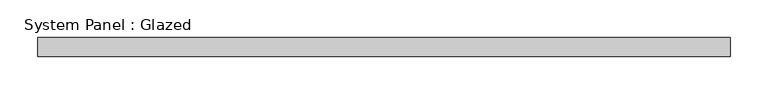
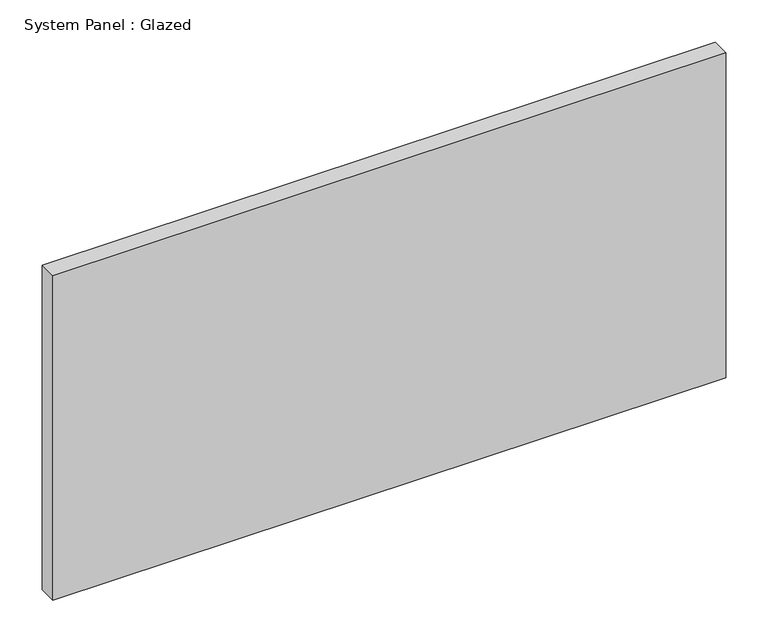
"""IFC4 building model written with IfcOpenShell, lengths in millimetres: plate geometry, System Panel : Glazed."""

from ifc_helpers import new_model, si_unit, origin, origin_with_axes, place, context, project, spatial, polyline, outline, extrude, source, transform, mapped, element, save


def system_panel_glazed_31531e99(model_context):
    return source(origin(), model_context, "Body", "SweptSolid", [
        extrude(outline(polyline([(460.375, 19.05), (-460.375, 19.05), (-460.375, 44.45), (460.375, 44.45), (460.375, 19.05)])), origin_with_axes(), (0.0, 0.0, 1.0), 469.9),
    ])


if __name__ == "__main__":
    model = new_model("IFC4")
    model_context = context("Model", 3, world=origin())
    ifc_project = project(units=[si_unit("LENGTHUNIT", "METRE", prefix="MILLI")], contexts=[model_context])
    site = spatial("IfcSite", under=ifc_project)
    building = spatial("IfcBuilding", under=site)
    placement = place(None, origin())
    system_panel_glazed_shape = system_panel_glazed_31531e99(model_context)
    element("IfcPlate", 1, ObjectType="System Panel : Glazed", at=placement, inside=building, context=model_context, shape_type="MappedRepresentation", body=[
        mapped(system_panel_glazed_shape, transform((0.0, 0.0, 0.0), x_axis=(1.0, 0.0, 0.0), y_axis=(0.0, 1.0, 0.0), z_axis=(0.0, 0.0, 1.0))),
    ])
    save(model, "model.ifc")

# Revit data of these elements
# Type "System Panel : Glazed"
#   Construction Type Id = "GSP4R"
#   Analytic Construction = "1/8 in Pilkington single glazing"
#   Visual Light Transmittance = 0.9
#   Solar Heat Gain Coefficient = 0.86
#   Heat Transfer Coefficient (U) = 1.18115 BTU/(h·ft²·°F)
#   Define Thermal Properties by = 1
# Element 1 (IfcPlate, "System Panel : Glazed")
#   Materials on its faces: "Glass"
# Materials
#   "Glass": class "Glass", colour RGB 0 128 192, transparency 0.75, Description = "Soda Lime Glass", Cost = 0
